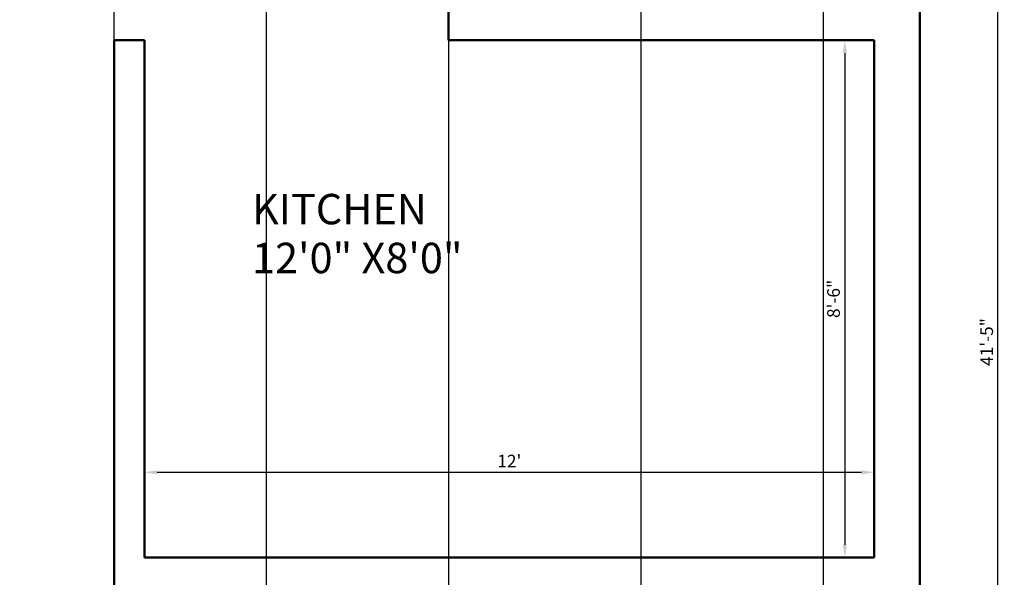
# Model space of a CAD drawing. Units: inches. Extents: x 2385 to 2740, y 1752 to 2305.
# Tile 11 of 15: x 2535 to 2729, y 1981 to 2091. Entities that reach past the tile are written whole.
import ezdxf

# ---------------------------------------------------------------- set-up
doc = ezdxf.new("R2010")
doc.units = ezdxf.units.IN
for name, color, linetype, lineweight in [('A-ANNO-DIMS', 2, 'Continuous', 18), ('A-AREA-IDEN', 7, 'Continuous', 25), ('A-WALL', 7, 'Continuous', 50)]:
    doc.layers.add(name, color=color, linetype=linetype, lineweight=lineweight)
doc.styles.get("Standard").update_dxf_attribs({"font": 'arial.ttf'})
doc.dimstyles.new('Copy of ISO-25', dxfattribs={"dimtxt": 2.5, "dimasz": 2.5, "dimexe": 1.25, "dimexo": 0.625, "dimtad": 1, "dimdec": 1, "dimlunit": 4, "dimtxsty": 'Standard', "dimcen": 2.5, "dimadec": 0, "dimazin": 0, "dimtfac": 1, "dimtdec": 1, "dimtmove": 0, "dimatfit": 3, "dimfxl": 1, "dimarcsym": 0})

# ---------------------------------------------------------------- blocks, each defined once
blk = doc.blocks.new('*D14')
at = {"layer": 'A-ANNO-DIMS', "color": 0, "lineweight": -2, "transparency": 16777216}
for p, q in [((2559.25, 1985.59), (2559.25, 2003.02)), ((2561.75, 2001.77), (2700.75, 2001.77)), ((2703.25, 1985.59), (2703.25, 2003.02))]:
    blk.add_line(p, q, dxfattribs=at)
at = {"layer": 'A-ANNO-DIMS', "color": 0, "transparency": 16777216}
for points in [[(2561.75, 2002.19), (2561.75, 2001.35), (2559.25, 2001.77)], [(2700.75, 2002.19), (2700.75, 2001.35), (2703.25, 2001.77)]]:
    blk.add_solid(points, dxfattribs=at)
at = {"layer": 'Defpoints', "color": 0, "transparency": 16777216}
for p in [(2703.25, 2001.77), (2559.25, 1984.97), (2703.25, 1984.97)]:
    blk.add_point(p, dxfattribs=at)
at = {"layer": 'A-ANNO-DIMS', "color": 0, "transparency": 16777216, "insert": (2631.25, 2003.65), "char_height": 2.5, "attachment_point": 5}
blk.add_mtext("12'", dxfattribs=at)
blk = doc.blocks.new('*D15')
at = {"layer": 'A-ANNO-DIMS', "color": 0, "lineweight": -2, "transparency": 16777216}
for p, q in [((2702.62, 2086.97), (2696.21, 2086.97)), ((2697.46, 2084.47), (2697.46, 1987.47)), ((2702.62, 1984.97), (2696.21, 1984.97))]:
    blk.add_line(p, q, dxfattribs=at)
at = {"layer": 'A-ANNO-DIMS', "color": 0, "transparency": 16777216}
for points in [[(2697.04, 2084.47), (2697.87, 2084.47), (2697.46, 2086.97)], [(2697.04, 1987.47), (2697.87, 1987.47), (2697.46, 1984.97)]]:
    blk.add_solid(points, dxfattribs=at)
at = {"layer": 'Defpoints', "color": 0, "transparency": 16777216}
for p in [(2703.25, 2086.97), (2697.46, 1984.97), (2703.25, 1984.97)]:
    blk.add_point(p, dxfattribs=at)
at = {"layer": 'A-ANNO-DIMS', "color": 0, "transparency": 16777216, "insert": (2695.55, 2035.97), "char_height": 2.5, "attachment_point": 5, "rotation": 90}
blk.add_mtext('8\'-6"', dxfattribs=at)
blk = doc.blocks.new('*D25')
at = {"layer": 'A-ANNO-DIMS', "color": 0, "lineweight": -2, "transparency": 16777216}
for p, q in [((2712.87, 2275.97), (2728.93, 2275.97)), ((2727.68, 1781.47), (2727.68, 2273.47)), ((2712.87, 1778.97), (2728.93, 1778.97))]:
    blk.add_line(p, q, dxfattribs=at)
at = {"layer": 'A-ANNO-DIMS', "color": 0, "transparency": 16777216}
for points in [[(2727.26, 2273.47), (2728.09, 2273.47), (2727.68, 2275.97)], [(2727.26, 1781.47), (2728.09, 1781.47), (2727.68, 1778.97)]]:
    blk.add_solid(points, dxfattribs=at)
at = {"layer": 'Defpoints', "color": 0, "transparency": 16777216}
for p in [(2712.25, 2275.97), (2727.68, 2275.97), (2712.25, 1778.97)]:
    blk.add_point(p, dxfattribs=at)
at = {"layer": 'A-ANNO-DIMS', "color": 0, "transparency": 16777216, "insert": (2725.77, 2027.47), "char_height": 2.5, "attachment_point": 5, "rotation": 90}
blk.add_mtext('41\'-5"', dxfattribs=at)
blk = doc.blocks.new('*D43')
at = {"layer": 'A-ANNO-DIMS', "color": 0, "lineweight": -2, "transparency": 16777216}
for p, q in [((2657.25, 1863.59), (2657.25, 2302.84)), ((2693.25, 1863.59), (2693.25, 2302.84)), ((2659.75, 2301.59), (2690.75, 2301.59))]:
    blk.add_line(p, q, dxfattribs=at)
at = {"layer": 'A-ANNO-DIMS', "color": 0, "transparency": 16777216}
for points in [[(2659.75, 2302), (2659.75, 2301.17), (2657.25, 2301.59)], [(2690.75, 2302), (2690.75, 2301.17), (2693.25, 2301.59)]]:
    blk.add_solid(points, dxfattribs=at)
at = {"layer": 'Defpoints', "color": 0, "transparency": 16777216}
for p in [(2693.25, 2301.59), (2657.25, 1862.97), (2693.25, 1862.97)]:
    blk.add_point(p, dxfattribs=at)
at = {"layer": 'A-ANNO-DIMS', "color": 0, "transparency": 16777216, "insert": (2675.25, 2303.49), "char_height": 2.5, "attachment_point": 5}
blk.add_mtext('3\'-0"', dxfattribs=at)
blk = doc.blocks.new('*D44')
at = {"layer": 'A-ANNO-DIMS', "color": 0, "lineweight": -2, "transparency": 16777216}
for p, q in [((2583.25, 2140.34), (2583.25, 1752.1)), ((2619.25, 2140.34), (2619.25, 1752.1)), ((2585.75, 1753.35), (2616.75, 1753.35))]:
    blk.add_line(p, q, dxfattribs=at)
at = {"layer": 'A-ANNO-DIMS', "color": 0, "transparency": 16777216}
for points in [[(2585.75, 1753.77), (2585.75, 1752.94), (2583.25, 1753.35)], [(2616.75, 1753.77), (2616.75, 1752.94), (2619.25, 1753.35)]]:
    blk.add_solid(points, dxfattribs=at)
at = {"layer": 'Defpoints', "color": 0, "transparency": 16777216}
for p in [(2583.25, 2140.97), (2619.25, 2140.97), (2619.25, 1753.35)]:
    blk.add_point(p, dxfattribs=at)
at = {"layer": 'A-ANNO-DIMS', "color": 0, "transparency": 16777216, "insert": (2601.25, 1755.25), "char_height": 2.5, "attachment_point": 5}
blk.add_mtext('3\'-0"', dxfattribs=at)
blk = doc.blocks.new('*D48')
at = {"layer": 'A-ANNO-DIMS', "color": 0, "lineweight": -2, "transparency": 16777216}
for p, q in [((2517.25, 1916.59), (2517.25, 2302.84)), ((2553.25, 1916.59), (2553.25, 2302.84)), ((2519.75, 2301.59), (2550.75, 2301.59))]:
    blk.add_line(p, q, dxfattribs=at)
at = {"layer": 'A-ANNO-DIMS', "color": 0, "transparency": 16777216}
for points in [[(2519.75, 2302), (2519.75, 2301.17), (2517.25, 2301.59)], [(2550.75, 2302), (2550.75, 2301.17), (2553.25, 2301.59)]]:
    blk.add_solid(points, dxfattribs=at)
at = {"layer": 'Defpoints', "color": 0, "transparency": 16777216}
for p in [(2553.25, 2301.59), (2517.25, 1915.97), (2553.25, 1915.97)]:
    blk.add_point(p, dxfattribs=at)
at = {"layer": 'A-ANNO-DIMS', "color": 0, "transparency": 16777216, "insert": (2535.25, 2303.49), "char_height": 2.5, "attachment_point": 5}
blk.add_mtext('3\'-0"', dxfattribs=at)

msp = doc.modelspace()

# ---------------------------------------------------------------- linework, layer by layer
at = {"layer": 'A-WALL'}
for p, q in [((2712.25, 2275.97), (2712.25, 1778.97)), ((2712.25, 2134.97), (2712.25, 2086.97)), ((2619.25, 2092.97), (2619.25, 2086.97)), ((2559.25, 2086.97), (2553.25, 2086.97)), ((2553.25, 2086.97), (2553.25, 1984.97)), ((2559.25, 2061.96), (2559.25, 2086.97)), ((2619.25, 2086.97), (2703.25, 2086.97)), ((2643.25, 2086.97), (2652.25, 2086.97)), ((2703.25, 2086.97), (2703.25, 2080.97)), ((2712.25, 2086.97), (2712.25, 2080.97)), ((2703.25, 2080.97), (2703.25, 1984.97)), ((2703.25, 2080.97), (2703.25, 1984.97)), ((2712.25, 2080.97), (2712.25, 1984.97)), ((2559.25, 1984.97), (2559.25, 2061.96)), ((2553.25, 1984.97), (2553.25, 1978.97)), ((2703.25, 1984.97), (2559.25, 1984.97)), ((2712.25, 1984.97), (2712.25, 1978.97))]:
    msp.add_line(p, q, dxfattribs=at)

# ---------------------------------------------------------------- texts
at = {"layer": 'A-AREA-IDEN'}
for s, p in [('KITCHEN', (2580.47, 2050.68)), ('12\'0" X8\'0"', (2580.47, 2041.04))]:
    msp.add_text(s, height=6, dxfattribs=at).set_placement(p)

# ---------------------------------------------------------------- dimensions: what is measured, and where the dimension line sits
at = {"layer": 'A-ANNO-DIMS'}
for base, p1, p2, override, picture, middle in [((2553.25, 2301.59), (2517.25, 1915.97), (2553.25, 1915.97), {"dimdec": 1, "dimlfac": 1, "dimrnd": 0, "dimzin": 1, "dimdsep": 46, "dimlunit": 4, "dimfrac": 2}, '*D48', (2535.25, 2303.49)), ((2693.25, 2301.59), (2657.25, 1862.97), (2693.25, 1862.97), {"dimdec": 1, "dimlfac": 1, "dimrnd": 0, "dimzin": 1, "dimdsep": 46, "dimlunit": 4, "dimfrac": 2}, '*D43', (2675.25, 2303.49)), ((2619.25, 1753.35), (2583.25, 2140.97), (2619.25, 2140.97), {"dimdec": 1, "dimlfac": 1, "dimrnd": 0, "dimzin": 1, "dimdsep": 46, "dimlunit": 4, "dimfrac": 2}, '*D44', (2601.25, 1755.25)), ((2703.25, 2001.77), (2559.25, 1984.97), (2703.25, 1984.97), {"dimclrd": 0, "dimclre": 0, "dimclrt": 0}, '*D14', (2631.25, 2003.65))]:
    dim = msp.add_linear_dim(base=base, p1=p1, p2=p2, dimstyle='Copy of ISO-25', override=override, dxfattribs=at)
    dim.commit()
    dim.dimension.update_dxf_attribs({"geometry": picture, "text_midpoint": middle})
for base, p1, p2, picture, middle in [((2727.68, 2275.97), (2712.25, 1778.97), (2712.25, 2275.97), '*D25', (2725.77, 2027.47)), ((2697.46, 1984.97), (2703.25, 2086.97), (2703.25, 1984.97), '*D15', (2695.55, 2035.97))]:
    dim = msp.add_linear_dim(base=base, p1=p1, p2=p2, angle=90, dimstyle='Copy of ISO-25', override={"dimclrd": 0, "dimclre": 0, "dimclrt": 0}, dxfattribs=at)
    dim.commit()
    dim.dimension.update_dxf_attribs({"geometry": picture, "text_midpoint": middle})

doc.saveas('drawing.dxf')
